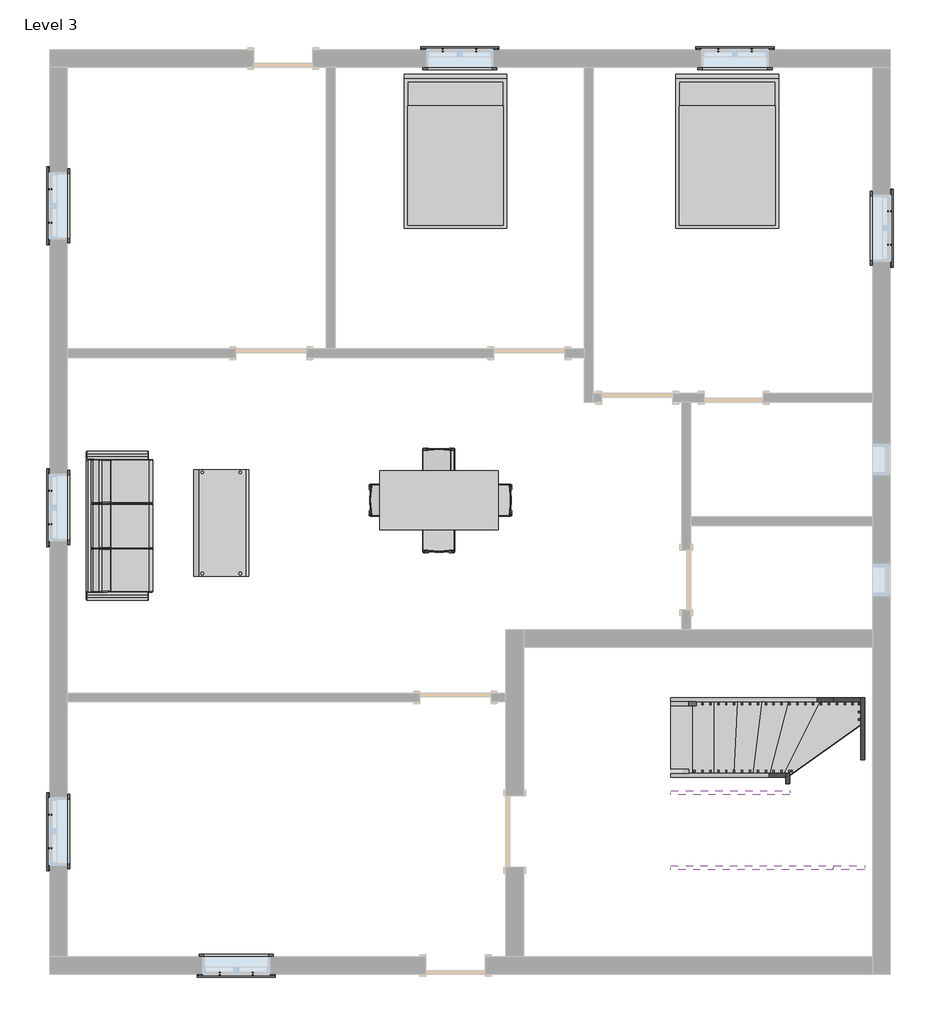
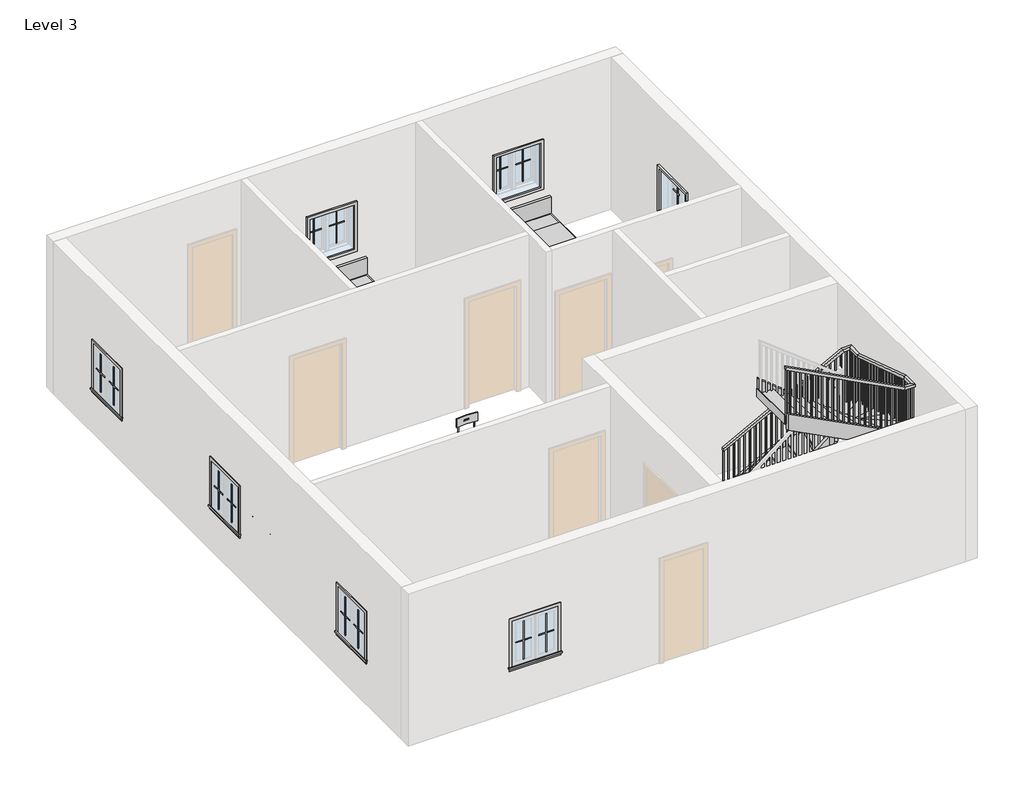
# One storey, part 2 of 2: 29 proxies, 8 members, 4 furniture elements, 1 railing, 1 stair flight.
"""IFC4 building model written with IfcOpenShell, lengths in millimetres."""

from ifc_helpers import new_model, si_unit, frame, origin, place, context, project, spatial, polyline, outline, extrude, faceted_brep, transform, mapped, element, save
from components import modern_coffee_table_17989_modern_coffee_table_17989_d3a860c8, muntin_pattern_2x2_muntin_pattern_2x2_b3fe6957, muntin_pattern_2x2_muntin_pattern_2x2_3e0ecaf2, trim_window_exterior_flat_with_sill_41619996, trim_window_interior_flat_picture_frame_51c85655, furniture_2fc85b74, furniture_29a9adb8, furniture_57072a26, bed_17739_bed_17739_15c61121, dining_table_w_chairs_11374_0cdfc61b, stair_flight_b9c50625

model = new_model("IFC4")

# Units and contexts
model_context = context("Model", 3, world=origin())
ifc_project = project(units=[si_unit("LENGTHUNIT", "METRE", prefix="MILLI")], contexts=[model_context])

# Site, building, storey
site = spatial("IfcSite", under=ifc_project)
building = spatial("IfcBuilding", under=site)
storey = spatial("IfcBuildingStorey", under=building, Name="Level 3", Elevation=3200.4)

# Proxies
placement = place(None, origin())
modern_coffee_table_17989_modern_coffee_table_17989_shape = modern_coffee_table_17989_modern_coffee_table_17989_d3a860c8(model_context)
element("IfcBuildingElementProxy", 1, Name="Modern_Coffee_Table_17989 : Modern_Coffee_Table_17989", ObjectType="Modern_Coffee_Table_17989 : Modern_Coffee_Table_17989", at=placement, inside=storey, context=model_context, shape_type="MappedRepresentation", body=[
    mapped(modern_coffee_table_17989_modern_coffee_table_17989_shape, transform((-4791.7841049, 1283.3840961, 3200.4), x_axis=(0.0, 1.0, 0.0), y_axis=(-1.0, 0.0, 0.0), z_axis=(0.0, 0.0, 1.0))),
])
muntin_pattern_2x2_muntin_pattern_2x2_shape = muntin_pattern_2x2_muntin_pattern_2x2_b3fe6957(model_context)
element("IfcBuildingElementProxy", 2, Name="Muntin Pattern_2x2 : Muntin Pattern_2x2", ObjectType="Muntin Pattern_2x2 : Muntin Pattern_2x2", at=placement, inside=storey, context=model_context, shape_type="MappedRepresentation", body=[
    mapped(muntin_pattern_2x2_muntin_pattern_2x2_shape, transform((-1586.7442864, 7129.6784997, 4184.65), x_axis=(1.0, 0.0, 0.0), y_axis=(0.0, 1.0, 0.0), z_axis=(0.0, 0.0, 1.0))),
])
element("IfcBuildingElementProxy", 3, Name="Muntin Pattern_2x2 : Muntin Pattern_2x2", ObjectType="Muntin Pattern_2x2 : Muntin Pattern_2x2", at=placement, inside=storey, context=model_context, shape_type="MappedRepresentation", body=[
    mapped(muntin_pattern_2x2_muntin_pattern_2x2_shape, transform((1952.1107136, 7129.6784997, 4184.65), x_axis=(1.0, 0.0, 0.0), y_axis=(0.0, 1.0, 0.0), z_axis=(0.0, 0.0, 1.0))),
])
element("IfcBuildingElementProxy", 4, Name="Muntin Pattern_2x2 : Muntin Pattern_2x2", ObjectType="Muntin Pattern_2x2 : Muntin Pattern_2x2", at=placement, inside=storey, context=model_context, shape_type="MappedRepresentation", body=[
    mapped(muntin_pattern_2x2_muntin_pattern_2x2_shape, transform((-6633.4067864, 4915.1159997, 4184.65), x_axis=(0.0, 1.0, 0.0), y_axis=(-1.0, 0.0, 0.0), z_axis=(0.0, 0.0, 1.0))),
])
element("IfcBuildingElementProxy", 5, Name="Muntin Pattern_2x2 : Muntin Pattern_2x2", ObjectType="Muntin Pattern_2x2 : Muntin Pattern_2x2", at=placement, inside=storey, context=model_context, shape_type="MappedRepresentation", body=[
    mapped(muntin_pattern_2x2_muntin_pattern_2x2_shape, transform((-6633.4067864, 1038.4409997, 4184.65), x_axis=(0.0, 1.0, 0.0), y_axis=(-1.0, 0.0, 0.0), z_axis=(0.0, 0.0, 1.0))),
])
element("IfcBuildingElementProxy", 6, Name="Muntin Pattern_2x2 : Muntin Pattern_2x2", ObjectType="Muntin Pattern_2x2 : Muntin Pattern_2x2", at=placement, inside=storey, context=model_context, shape_type="MappedRepresentation", body=[
    mapped(muntin_pattern_2x2_muntin_pattern_2x2_shape, transform((4152.7032136, 5057.9909997, 4184.65), x_axis=(0.0, -1.0, 0.0), y_axis=(1.0, 0.0, 0.0), z_axis=(0.0, 0.0, 1.0))),
])
element("IfcBuildingElementProxy", 7, Name="Muntin Pattern_2x2 : Muntin Pattern_2x2", ObjectType="Muntin Pattern_2x2 : Muntin Pattern_2x2", at=placement, inside=storey, context=model_context, shape_type="MappedRepresentation", body=[
    mapped(muntin_pattern_2x2_muntin_pattern_2x2_shape, transform((-6633.4067864, -3125.2540003, 4184.65), x_axis=(0.0, 1.0, 0.0), y_axis=(-1.0, 0.0, 0.0), z_axis=(0.0, 0.0, 1.0))),
])
element("IfcBuildingElementProxy", 8, Name="Muntin Pattern_2x2 : Muntin Pattern_2x2", ObjectType="Muntin Pattern_2x2 : Muntin Pattern_2x2", at=placement, inside=storey, context=model_context, shape_type="MappedRepresentation", body=[
    mapped(muntin_pattern_2x2_muntin_pattern_2x2_shape, transform((-4028.3192864, -4738.4715003, 4184.65), x_axis=(-1.0, 0.0, 0.0), y_axis=(0.0, -1.0, 0.0), z_axis=(0.0, 0.0, 1.0))),
])
muntin_pattern_2x2_muntin_pattern_2x2_2_shape = muntin_pattern_2x2_muntin_pattern_2x2_3e0ecaf2(model_context)
element("IfcBuildingElementProxy", 9, Name="Muntin Pattern_2x2 : Muntin Pattern_2x2", ObjectType="Muntin Pattern_2x2 : Muntin Pattern_2x2", at=placement, inside=storey, context=model_context, shape_type="MappedRepresentation", body=[
    mapped(muntin_pattern_2x2_muntin_pattern_2x2_2_shape, transform((-1158.1192864, 7129.6784997, 4184.65), x_axis=(-1.0, 0.0, 0.0), y_axis=(0.0, -1.0, 0.0), z_axis=(0.0, 0.0, 1.0))),
])
element("IfcBuildingElementProxy", 10, Name="Muntin Pattern_2x2 : Muntin Pattern_2x2", ObjectType="Muntin Pattern_2x2 : Muntin Pattern_2x2", at=placement, inside=storey, context=model_context, shape_type="MappedRepresentation", body=[
    mapped(muntin_pattern_2x2_muntin_pattern_2x2_2_shape, transform((2380.7357136, 7129.6784997, 4184.65), x_axis=(-1.0, 0.0, 0.0), y_axis=(0.0, -1.0, 0.0), z_axis=(0.0, 0.0, 1.0))),
])
element("IfcBuildingElementProxy", 11, Name="Muntin Pattern_2x2 : Muntin Pattern_2x2", ObjectType="Muntin Pattern_2x2 : Muntin Pattern_2x2", at=placement, inside=storey, context=model_context, shape_type="MappedRepresentation", body=[
    mapped(muntin_pattern_2x2_muntin_pattern_2x2_2_shape, transform((-6633.4067864, 5343.7409997, 4184.65), x_axis=(0.0, -1.0, 0.0), y_axis=(1.0, 0.0, 0.0), z_axis=(0.0, 0.0, 1.0))),
])
element("IfcBuildingElementProxy", 12, Name="Muntin Pattern_2x2 : Muntin Pattern_2x2", ObjectType="Muntin Pattern_2x2 : Muntin Pattern_2x2", at=placement, inside=storey, context=model_context, shape_type="MappedRepresentation", body=[
    mapped(muntin_pattern_2x2_muntin_pattern_2x2_2_shape, transform((-6633.4067864, 1467.0659997, 4184.65), x_axis=(0.0, -1.0, 0.0), y_axis=(1.0, 0.0, 0.0), z_axis=(0.0, 0.0, 1.0))),
])
element("IfcBuildingElementProxy", 13, Name="Muntin Pattern_2x2 : Muntin Pattern_2x2", ObjectType="Muntin Pattern_2x2 : Muntin Pattern_2x2", at=placement, inside=storey, context=model_context, shape_type="MappedRepresentation", body=[
    mapped(muntin_pattern_2x2_muntin_pattern_2x2_2_shape, transform((4152.7032136, 4629.3659997, 4184.65), x_axis=(0.0, 1.0, 0.0), y_axis=(-1.0, 0.0, 0.0), z_axis=(0.0, 0.0, 1.0))),
])
element("IfcBuildingElementProxy", 14, Name="Muntin Pattern_2x2 : Muntin Pattern_2x2", ObjectType="Muntin Pattern_2x2 : Muntin Pattern_2x2", at=placement, inside=storey, context=model_context, shape_type="MappedRepresentation", body=[
    mapped(muntin_pattern_2x2_muntin_pattern_2x2_2_shape, transform((-6633.4067864, -2696.6290003, 4184.65), x_axis=(0.0, -1.0, 0.0), y_axis=(1.0, 0.0, 0.0), z_axis=(0.0, 0.0, 1.0))),
])
element("IfcBuildingElementProxy", 15, Name="Muntin Pattern_2x2 : Muntin Pattern_2x2", ObjectType="Muntin Pattern_2x2 : Muntin Pattern_2x2", at=placement, inside=storey, context=model_context, shape_type="MappedRepresentation", body=[
    mapped(muntin_pattern_2x2_muntin_pattern_2x2_2_shape, transform((-4456.9442864, -4738.4715003, 4184.65), x_axis=(1.0, 0.0, 0.0), y_axis=(0.0, 1.0, 0.0), z_axis=(0.0, 0.0, 1.0))),
])
trim_window_exterior_flat_with_sill_shape = trim_window_exterior_flat_with_sill_41619996(model_context)
element("IfcBuildingElementProxy", 16, Name="Trim-Window-Exterior-Flat : with Sill", ObjectType="Trim-Window-Exterior-Flat : with Sill", at=placement, inside=storey, context=model_context, shape_type="MappedRepresentation", body=[
    mapped(trim_window_exterior_flat_with_sill_shape, transform((-1372.4317864, 7139.2034997, 5029.2), x_axis=(-1.0, 0.0, 0.0), y_axis=(0.0, 0.0, 1.0), z_axis=(0.0, 1.0, 0.0))),
])
element("IfcBuildingElementProxy", 17, Name="Trim-Window-Exterior-Flat : with Sill", ObjectType="Trim-Window-Exterior-Flat : with Sill", at=placement, inside=storey, context=model_context, shape_type="MappedRepresentation", body=[
    mapped(trim_window_exterior_flat_with_sill_shape, transform((2166.4232136, 7139.2034997, 5029.2), x_axis=(-1.0, 0.0, 0.0), y_axis=(0.0, 0.0, 1.0), z_axis=(0.0, 1.0, 0.0))),
])
element("IfcBuildingElementProxy", 18, Name="Trim-Window-Exterior-Flat : with Sill", ObjectType="Trim-Window-Exterior-Flat : with Sill", at=placement, inside=storey, context=model_context, shape_type="MappedRepresentation", body=[
    mapped(trim_window_exterior_flat_with_sill_shape, transform((-6642.9317864, 5129.4284997, 5029.2), x_axis=(0.0, -1.0, 0.0), y_axis=(0.0, 0.0, 1.0), z_axis=(-1.0, 0.0, 0.0))),
])
element("IfcBuildingElementProxy", 19, Name="Trim-Window-Exterior-Flat : with Sill", ObjectType="Trim-Window-Exterior-Flat : with Sill", at=placement, inside=storey, context=model_context, shape_type="MappedRepresentation", body=[
    mapped(trim_window_exterior_flat_with_sill_shape, transform((-6642.9317864, 1252.7534997, 5029.2), x_axis=(0.0, -1.0, 0.0), y_axis=(0.0, 0.0, 1.0), z_axis=(-1.0, 0.0, 0.0))),
])
element("IfcBuildingElementProxy", 20, Name="Trim-Window-Exterior-Flat : with Sill", ObjectType="Trim-Window-Exterior-Flat : with Sill", at=placement, inside=storey, context=model_context, shape_type="MappedRepresentation", body=[
    mapped(trim_window_exterior_flat_with_sill_shape, transform((4162.2282136, 4843.6784997, 5029.2), x_axis=(0.0, 1.0, 0.0), y_axis=(0.0, 0.0, 1.0), z_axis=(1.0, 0.0, 0.0))),
])
element("IfcBuildingElementProxy", 21, Name="Trim-Window-Exterior-Flat : with Sill", ObjectType="Trim-Window-Exterior-Flat : with Sill", at=placement, inside=storey, context=model_context, shape_type="MappedRepresentation", body=[
    mapped(trim_window_exterior_flat_with_sill_shape, transform((-6642.9317864, -2910.9415003, 5029.2), x_axis=(0.0, -1.0, 0.0), y_axis=(0.0, 0.0, 1.0), z_axis=(-1.0, 0.0, 0.0))),
])
element("IfcBuildingElementProxy", 22, Name="Trim-Window-Exterior-Flat : with Sill", ObjectType="Trim-Window-Exterior-Flat : with Sill", at=placement, inside=storey, context=model_context, shape_type="MappedRepresentation", body=[
    mapped(trim_window_exterior_flat_with_sill_shape, transform((-4242.6317864, -4747.9965003, 5029.2), x_axis=(1.0, 0.0, 0.0), y_axis=(0.0, 0.0, 1.0), z_axis=(0.0, -1.0, 0.0))),
])
trim_window_interior_flat_picture_frame_shape = trim_window_interior_flat_picture_frame_51c85655(model_context)
element("IfcBuildingElementProxy", 23, Name="Trim-Window-Interior-Flat : Picture Frame", ObjectType="Trim-Window-Interior-Flat : Picture Frame", at=placement, inside=storey, context=model_context, shape_type="MappedRepresentation", body=[
    mapped(trim_window_interior_flat_picture_frame_shape, transform((-1372.4317864, 6910.6034997, 5029.2), x_axis=(1.0, 0.0, 0.0), y_axis=(0.0, 0.0, 1.0), z_axis=(0.0, -1.0, 0.0))),
])
element("IfcBuildingElementProxy", 24, Name="Trim-Window-Interior-Flat : Picture Frame", ObjectType="Trim-Window-Interior-Flat : Picture Frame", at=placement, inside=storey, context=model_context, shape_type="MappedRepresentation", body=[
    mapped(trim_window_interior_flat_picture_frame_shape, transform((2166.4232136, 6910.6034997, 5029.2), x_axis=(1.0, 0.0, 0.0), y_axis=(0.0, 0.0, 1.0), z_axis=(0.0, -1.0, 0.0))),
])
element("IfcBuildingElementProxy", 25, Name="Trim-Window-Interior-Flat : Picture Frame", ObjectType="Trim-Window-Interior-Flat : Picture Frame", at=placement, inside=storey, context=model_context, shape_type="MappedRepresentation", body=[
    mapped(trim_window_interior_flat_picture_frame_shape, transform((-6414.3317864, 5129.4284997, 5029.2), x_axis=(0.0, 1.0, 0.0), y_axis=(0.0, 0.0, 1.0), z_axis=(1.0, 0.0, 0.0))),
])
element("IfcBuildingElementProxy", 26, Name="Trim-Window-Interior-Flat : Picture Frame", ObjectType="Trim-Window-Interior-Flat : Picture Frame", at=placement, inside=storey, context=model_context, shape_type="MappedRepresentation", body=[
    mapped(trim_window_interior_flat_picture_frame_shape, transform((-6414.3317864, 1252.7534997, 5029.2), x_axis=(0.0, 1.0, 0.0), y_axis=(0.0, 0.0, 1.0), z_axis=(1.0, 0.0, 0.0))),
])
element("IfcBuildingElementProxy", 27, Name="Trim-Window-Interior-Flat : Picture Frame", ObjectType="Trim-Window-Interior-Flat : Picture Frame", at=placement, inside=storey, context=model_context, shape_type="MappedRepresentation", body=[
    mapped(trim_window_interior_flat_picture_frame_shape, transform((3933.6282136, 4843.6784997, 5029.2), x_axis=(0.0, -1.0, 0.0), y_axis=(0.0, 0.0, 1.0), z_axis=(-1.0, 0.0, 0.0))),
])
element("IfcBuildingElementProxy", 28, Name="Trim-Window-Interior-Flat : Picture Frame", ObjectType="Trim-Window-Interior-Flat : Picture Frame", at=placement, inside=storey, context=model_context, shape_type="MappedRepresentation", body=[
    mapped(trim_window_interior_flat_picture_frame_shape, transform((-6414.3317864, -2910.9415003, 5029.2), x_axis=(0.0, 1.0, 0.0), y_axis=(0.0, 0.0, 1.0), z_axis=(1.0, 0.0, 0.0))),
])
element("IfcBuildingElementProxy", 29, Name="Trim-Window-Interior-Flat : Picture Frame", ObjectType="Trim-Window-Interior-Flat : Picture Frame", at=placement, inside=storey, context=model_context, shape_type="MappedRepresentation", body=[
    mapped(trim_window_interior_flat_picture_frame_shape, transform((-4242.6317864, -4519.3965003, 5029.2), x_axis=(-1.0, 0.0, 0.0), y_axis=(0.0, 0.0, 1.0), z_axis=(0.0, 1.0, 0.0))),
])

# Furniture
furniture_shape = furniture_2fc85b74(model_context)
furniture_2_shape = furniture_29a9adb8(model_context)
furniture_3_shape = furniture_57072a26(model_context)
element("IfcFurniture", 30, at=placement, inside=storey, context=model_context, shape_type="MappedRepresentation", body=[
    mapped(furniture_shape, transform((-5371.0104604, 1017.8034997, 3200.4), x_axis=(0.0, 1.0, 0.0), y_axis=(-1.0, 0.0, 0.0), z_axis=(0.0, 0.0, 1.0))),
    mapped(furniture_2_shape, transform((-5371.0104604, 1017.8034997, 3200.4), x_axis=(0.0, 1.0, 0.0), y_axis=(-1.0, 0.0, 0.0), z_axis=(0.0, 0.0, 1.0))),
    mapped(furniture_3_shape, transform((-5371.0104604, 1017.8034997, 3200.4), x_axis=(0.0, 1.0, 0.0), y_axis=(-1.0, 0.0, 0.0), z_axis=(0.0, 0.0, 1.0))),
])
bed_17739_bed_17739_shape = bed_17739_bed_17739_15c61121(model_context)
element("IfcFurniture", 31, ObjectType="Bed_17739 : Bed_17739", at=placement, inside=storey, context=model_context, shape_type="MappedRepresentation", body=[
    mapped(bed_17739_bed_17739_shape, transform((-1425.7717864, 5805.7034997, 3200.4), x_axis=(1.0, 0.0, 0.0), y_axis=(0.0, 1.0, 0.0), z_axis=(0.0, 0.0, 1.0))),
])
element("IfcFurniture", 32, ObjectType="Bed_17739 : Bed_17739", at=placement, inside=storey, context=model_context, shape_type="MappedRepresentation", body=[
    mapped(bed_17739_bed_17739_shape, transform((2066.7282136, 5805.7034997, 3200.4), x_axis=(1.0, 0.0, 0.0), y_axis=(0.0, 1.0, 0.0), z_axis=(0.0, 0.0, 1.0))),
])
dining_table_w_chairs_11374_shape = dining_table_w_chairs_11374_0cdfc61b(model_context)
element("IfcFurniture", 33, ObjectType="Dining_Table_w_Chairs_11374", at=placement, inside=storey, context=model_context, shape_type="MappedRepresentation", body=[
    mapped(dining_table_w_chairs_11374_shape, transform((-1657.0397106, 1252.0888157, 3200.4), x_axis=(1.0, 0.0, 0.0), y_axis=(0.0, 1.0, 0.0), z_axis=(0.0, 0.0, 1.0))),
])

# Members
element("IfcMember", 34, ObjectType="Stringer - 2\" Width", at=placement, inside=storey, context=model_context, shape_type="SweptSolid", body=[
    extrude(outline(polyline([(3430.039954, 1342.8282136), (3200.4, 1342.8282136), (3200.4, 1562.5905312), (4162.900629, 3430.2454053), (4505.7956453, 3430.2454053), (3430.039954, 1342.8282136)])), frame((0.0, -1245.3365003, 0.0), z_axis=(0.0, 1.0, 0.0), x_axis=(0.0, 0.0, 1.0)), (0.0, 0.0, 1.0), 50.8),
])
element("IfcMember", 35, ObjectType="Stringer - 2\" Width", at=placement, inside=storey, context=model_context, shape_type="SweptSolid", body=[
    extrude(outline(polyline([(3430.2454053, -1245.3365003), (3430.2454053, -1194.5365003), (3784.9599055, -1194.5365003), (3784.9599055, -1245.3365003), (3430.2454053, -1245.3365003)])), frame((0.0, 0.0, 4162.900629), z_axis=(0.0, 0.0, 1.0), x_axis=(1.0, 0.0, 0.0)), (0.0, 0.0, 1.0), 342.8950162),
])
element("IfcMember", 36, ObjectType="Stringer - 2\" Width", at=placement, inside=storey, context=model_context, shape_type="SweptSolid", body=[
    extrude(outline(polyline([(-1194.5365003, 4489.4952212), (-1194.5365003, 4200.9956453), (-1364.0589833, 4200.9956453), (-3353.5365003, 4839.3682298), (-3353.5365003, 5170.3972697), (-3316.5563831, 5170.3972697), (-1194.5365003, 4489.4952212)])), frame((3784.9599055, 0.0, 0.0), z_axis=(1.0, 0.0, 0.0), x_axis=(0.0, 1.0, 0.0)), (0.0, 0.0, 1.0), 50.8),
])
element("IfcMember", 37, ObjectType="Stringer - 2\" Width", at=placement, inside=storey, context=model_context, shape_type="SweptSolid", body=[
    extrude(outline(polyline([(3835.7599055, -3353.5365003), (3835.7599055, -3404.3365003), (3430.2454053, -3404.3365003), (3430.2454053, -3353.5365003), (3835.7599055, -3353.5365003)])), frame((0.0, 0.0, 4850.2904473), z_axis=(0.0, 0.0, 1.0), x_axis=(1.0, 0.0, 0.0)), (0.0, 0.0, 1.0), 320.1068224),
])
element("IfcMember", 38, ObjectType="Stringer - 2\" Width", at=placement, inside=storey, context=model_context, shape_type="SweptSolid", body=[
    extrude(outline(polyline([(4850.2904473, 3430.2454053), (5170.3972697, 3430.2454053), (6246.1529609, 1342.8282136), (5926.0461385, 1342.8282136), (4850.2904473, 3430.2454053)])), frame((0.0, -3404.3365003, 0.0), z_axis=(0.0, 1.0, 0.0), x_axis=(0.0, 0.0, 1.0)), (0.0, 0.0, 1.0), 50.8),
])
element("IfcMember", 39, ObjectType="Stringer - 2\" Width", at=placement, inside=storey, context=model_context, shape_type="SweptSolid", body=[
    extrude(outline(polyline([(3376.5764461, 1342.8282136), (3200.4, 1342.8282136), (3200.4, 1609.0898582), (4187.5410923, 2819.7599055), (4580.818648, 2819.7599055), (3376.5764461, 1342.8282136)])), frame((0.0, -2210.5365003, 0.0), z_axis=(0.0, 1.0, 0.0), x_axis=(0.0, 0.0, 1.0)), (0.0, 0.0, 1.0), 50.8),
])
element("IfcMember", 40, ObjectType="Stringer - 2\" Width", at=placement, inside=storey, context=model_context, shape_type="SweptSolid", body=[
    extrude(outline(polyline([(-2159.7365003, 4773.6682978), (-2159.7365003, 4228.9617647), (-2193.9787177, 4228.9617647), (-2388.3365003, 4560.865107), (-2388.3365003, 5126.5409689), (-2366.3736178, 5126.5409689), (-2159.7365003, 4773.6682978)])), frame((2819.7599055, 0.0, 0.0), z_axis=(1.0, 0.0, 0.0), x_axis=(0.0, 1.0, 0.0)), (0.0, 0.0, 1.0), 50.8),
])
element("IfcMember", 41, ObjectType="Stringer - 2\" Width", at=placement, inside=storey, context=model_context, shape_type="SweptSolid", body=[
    extrude(outline(polyline([(4733.2634131, 2870.5599055), (5126.5409689, 2870.5599055), (6372.2038432, 1342.8282136), (5978.9262875, 1342.8282136), (4733.2634131, 2870.5599055)])), frame((0.0, -2439.1365003, 0.0), z_axis=(0.0, 1.0, 0.0), x_axis=(0.0, 0.0, 1.0)), (0.0, 0.0, 1.0), 50.8),
])

# Railing
element("IfcRailing", 42, ObjectType="Handrail - Rectangular", at=placement, inside=storey, context=model_context, shape_type="SolidModel", body=[
    faceted_brep([(1342.8282136, -1245.3365003, 4284.1333333), (1342.8282136, -1245.3365003, 4226.6742652), (1342.8282136, -1296.1365003, 4226.6742652), (1342.8282136, -1296.1365003, 4284.1333333), (3600.5532757, -1245.3365003, 5477.4239201), (3613.1523402, -1245.3365003, 5426.6239201), (3613.1523402, -1296.1365003, 5426.6239201), (3600.5532757, -1296.1365003, 5477.4239201), (3784.9599055, -1245.3365003, 5477.4239201), (3784.9599055, -1245.3365003, 5426.6239201), (3734.1599055, -1296.1365003, 5426.6239201), (3734.1599055, -1296.1365003, 5477.4239201), (3784.9599055, -1532.6483825, 5477.4239201), (3784.9599055, -1540.5989586, 5426.6239201), (3734.1599055, -1540.5989586, 5426.6239201), (3734.1599055, -1532.6483825, 5477.4239201), (3784.9599055, -3066.2246182, 5969.5094132), (3784.9599055, -3074.1751943, 5918.7094132), (3734.1599055, -3074.1751943, 5918.7094132), (3734.1599055, -3066.2246182, 5969.5094132), (3784.9599055, -3353.5365003, 5969.5094132), (3784.9599055, -3353.5365003, 5918.7094132), (3734.1599055, -3302.7365003, 5918.7094132), (3734.1599055, -3302.7365003, 5969.5094132), (3600.5532757, -3353.5365003, 5969.5094132), (3587.9542112, -3353.5365003, 5918.7094132), (3587.9542112, -3302.7365003, 5918.7094132), (3600.5532757, -3302.7365003, 5969.5094132), (1342.8282136, -3353.5365003, 7162.8), (1342.8282136, -3302.7365003, 7162.8), (1342.8282136, -3302.7365003, 7105.3409318), (1342.8282136, -3353.5365003, 7105.3409318)], [[[0, 1, 2, 3]], [[1, 0, 4, 5]], [[2, 1, 5, 6]], [[3, 2, 6, 7]], [[0, 3, 7, 4]], [[5, 4, 8, 9]], [[6, 5, 9, 10]], [[7, 6, 10, 11]], [[4, 7, 11, 8]], [[9, 8, 12, 13]], [[10, 9, 13, 14]], [[11, 10, 14, 15]], [[8, 11, 15, 12]], [[13, 12, 16, 17]], [[14, 13, 17, 18]], [[15, 14, 18, 19]], [[12, 15, 19, 16]], [[17, 16, 20, 21]], [[18, 17, 21, 22]], [[19, 18, 22, 23]], [[16, 19, 23, 20]], [[21, 20, 24, 25]], [[22, 21, 25, 26]], [[23, 22, 26, 27]], [[20, 23, 27, 24]], [[28, 29, 30, 31]], [[25, 24, 28, 31]], [[26, 25, 31, 30]], [[27, 26, 30, 29]], [[24, 27, 29, 28]]]),
    extrude(outline(polyline([(7068.1284102, 1413.2349055), (6079.0666667, 1413.2349055), (6079.0666667, 1432.2849055), (7058.0597858, 1432.2849055), (7068.1284102, 1413.2349055)])), frame((0.0, -3337.6615003, 0.0), z_axis=(0.0, 1.0, 0.0), x_axis=(0.0, 0.0, 1.0)), (0.0, 0.0, 1.0), 19.05),
    extrude(outline(polyline([(7014.42908, 1514.8349055), (6079.0666667, 1514.8349055), (6079.0666667, 1533.8849055), (7004.3604556, 1533.8849055), (7014.42908, 1514.8349055)])), frame((0.0, -3337.6615003, 0.0), z_axis=(0.0, 1.0, 0.0), x_axis=(0.0, 0.0, 1.0)), (0.0, 0.0, 1.0), 19.05),
    extrude(outline(polyline([(6960.7297498, 1616.4349055), (5909.7333333, 1616.4349055), (5909.7333333, 1635.4849055), (6950.6611254, 1635.4849055), (6960.7297498, 1616.4349055)])), frame((0.0, -3337.6615003, 0.0), z_axis=(0.0, 1.0, 0.0), x_axis=(0.0, 0.0, 1.0)), (0.0, 0.0, 1.0), 19.05),
    extrude(outline(polyline([(6907.0304196, 1718.0349055), (5909.7333333, 1718.0349055), (5909.7333333, 1737.0849055), (6896.9617952, 1737.0849055), (6907.0304196, 1718.0349055)])), frame((0.0, -3337.6615003, 0.0), z_axis=(0.0, 1.0, 0.0), x_axis=(0.0, 0.0, 1.0)), (0.0, 0.0, 1.0), 19.05),
    extrude(outline(polyline([(6853.3310894, 1819.6349055), (5909.7333333, 1819.6349055), (5909.7333333, 1838.6849055), (6843.262465, 1838.6849055), (6853.3310894, 1819.6349055)])), frame((0.0, -3337.6615003, 0.0), z_axis=(0.0, 1.0, 0.0), x_axis=(0.0, 0.0, 1.0)), (0.0, 0.0, 1.0), 19.05),
    extrude(outline(polyline([(6799.6317592, 1921.2349055), (5740.4, 1921.2349055), (5740.4, 1940.2849055), (6789.5631348, 1940.2849055), (6799.6317592, 1921.2349055)])), frame((0.0, -3337.6615003, 0.0), z_axis=(0.0, 1.0, 0.0), x_axis=(0.0, 0.0, 1.0)), (0.0, 0.0, 1.0), 19.05),
    extrude(outline(polyline([(6745.932429, 2022.8349055), (5740.4, 2022.8349055), (5740.4, 2041.8849055), (6735.8638046, 2041.8849055), (6745.932429, 2022.8349055)])), frame((0.0, -3337.6615003, 0.0), z_axis=(0.0, 1.0, 0.0), x_axis=(0.0, 0.0, 1.0)), (0.0, 0.0, 1.0), 19.05),
    extrude(outline(polyline([(6692.2330988, 2124.4349055), (5740.4, 2124.4349055), (5740.4, 2143.4849055), (6682.1644744, 2143.4849055), (6692.2330988, 2124.4349055)])), frame((0.0, -3337.6615003, 0.0), z_axis=(0.0, 1.0, 0.0), x_axis=(0.0, 0.0, 1.0)), (0.0, 0.0, 1.0), 19.05),
    extrude(outline(polyline([(6638.5337686, 2226.0349055), (5571.0666667, 2226.0349055), (5571.0666667, 2245.0849055), (6628.4651442, 2245.0849055), (6638.5337686, 2226.0349055)])), frame((0.0, -3337.6615003, 0.0), z_axis=(0.0, 1.0, 0.0), x_axis=(0.0, 0.0, 1.0)), (0.0, 0.0, 1.0), 19.05),
    extrude(outline(polyline([(6584.8344384, 2327.6349055), (5571.0666667, 2327.6349055), (5571.0666667, 2346.6849055), (6574.765814, 2346.6849055), (6584.8344384, 2327.6349055)])), frame((0.0, -3337.6615003, 0.0), z_axis=(0.0, 1.0, 0.0), x_axis=(0.0, 0.0, 1.0)), (0.0, 0.0, 1.0), 19.05),
    extrude(outline(polyline([(6531.1351082, 2429.2349055), (5571.0666667, 2429.2349055), (5571.0666667, 2448.2849055), (6521.0664838, 2448.2849055), (6531.1351082, 2429.2349055)])), frame((0.0, -3337.6615003, 0.0), z_axis=(0.0, 1.0, 0.0), x_axis=(0.0, 0.0, 1.0)), (0.0, 0.0, 1.0), 19.05),
    extrude(outline(polyline([(6477.435778, 2530.8349055), (5401.7333333, 2530.8349055), (5401.7333333, 2549.8849055), (6467.3671536, 2549.8849055), (6477.435778, 2530.8349055)])), frame((0.0, -3337.6615003, 0.0), z_axis=(0.0, 1.0, 0.0), x_axis=(0.0, 0.0, 1.0)), (0.0, 0.0, 1.0), 19.05),
    extrude(outline(polyline([(6423.7364478, 2632.4349055), (5401.7333333, 2632.4349055), (5401.7333333, 2651.4849055), (6413.6678234, 2651.4849055), (6423.7364478, 2632.4349055)])), frame((0.0, -3337.6615003, 0.0), z_axis=(0.0, 1.0, 0.0), x_axis=(0.0, 0.0, 1.0)), (0.0, 0.0, 1.0), 19.05),
    extrude(outline(polyline([(6370.0371176, 2734.0349055), (5401.7333333, 2734.0349055), (5401.7333333, 2753.0849055), (6359.9684932, 2753.0849055), (6370.0371176, 2734.0349055)])), frame((0.0, -3337.6615003, 0.0), z_axis=(0.0, 1.0, 0.0), x_axis=(0.0, 0.0, 1.0)), (0.0, 0.0, 1.0), 19.05),
    extrude(outline(polyline([(6316.3377874, 2835.6349055), (5401.7333333, 2835.6349055), (5401.7333333, 2854.6849055), (6306.269163, 2854.6849055), (6316.3377874, 2835.6349055)])), frame((0.0, -3337.6615003, 0.0), z_axis=(0.0, 1.0, 0.0), x_axis=(0.0, 0.0, 1.0)), (0.0, 0.0, 1.0), 19.05),
    extrude(outline(polyline([(6262.6384572, 2937.2349055), (5232.4, 2937.2349055), (5232.4, 2956.2849055), (6252.5698328, 2956.2849055), (6262.6384572, 2937.2349055)])), frame((0.0, -3337.6615003, 0.0), z_axis=(0.0, 1.0, 0.0), x_axis=(0.0, 0.0, 1.0)), (0.0, 0.0, 1.0), 19.05),
    extrude(outline(polyline([(6208.939127, 3038.8349055), (5232.4, 3038.8349055), (5232.4, 3057.8849055), (6198.8705026, 3057.8849055), (6208.939127, 3038.8349055)])), frame((0.0, -3337.6615003, 0.0), z_axis=(0.0, 1.0, 0.0), x_axis=(0.0, 0.0, 1.0)), (0.0, 0.0, 1.0), 19.05),
    extrude(outline(polyline([(6155.2397968, 3140.4349055), (5232.4, 3140.4349055), (5232.4, 3159.4849055), (6145.1711724, 3159.4849055), (6155.2397968, 3140.4349055)])), frame((0.0, -3337.6615003, 0.0), z_axis=(0.0, 1.0, 0.0), x_axis=(0.0, 0.0, 1.0)), (0.0, 0.0, 1.0), 19.05),
    extrude(outline(polyline([(6101.5404666, 3242.0349055), (5232.4, 3242.0349055), (5232.4, 3261.0849055), (6091.4718422, 3261.0849055), (6101.5404666, 3242.0349055)])), frame((0.0, -3337.6615003, 0.0), z_axis=(0.0, 1.0, 0.0), x_axis=(0.0, 0.0, 1.0)), (0.0, 0.0, 1.0), 19.05),
    extrude(outline(polyline([(6047.8411364, 3343.6349055), (5063.0666667, 3343.6349055), (5063.0666667, 3362.6849055), (6037.772512, 3362.6849055), (6047.8411364, 3343.6349055)])), frame((0.0, -3337.6615003, 0.0), z_axis=(0.0, 1.0, 0.0), x_axis=(0.0, 0.0, 1.0)), (0.0, 0.0, 1.0), 19.05),
    extrude(outline(polyline([(5994.1418062, 3445.2349055), (5063.0666667, 3445.2349055), (5063.0666667, 3464.2849055), (5984.0731818, 3464.2849055), (5994.1418062, 3445.2349055)])), frame((0.0, -3337.6615003, 0.0), z_axis=(0.0, 1.0, 0.0), x_axis=(0.0, 0.0, 1.0)), (0.0, 0.0, 1.0), 19.05),
    extrude(outline(polyline([(5940.442476, 3546.8349055), (5063.0666667, 3546.8349055), (5063.0666667, 3565.8849055), (5930.3738516, 3565.8849055), (5940.442476, 3546.8349055)])), frame((0.0, -3337.6615003, 0.0), z_axis=(0.0, 1.0, 0.0), x_axis=(0.0, 0.0, 1.0)), (0.0, 0.0, 1.0), 19.05),
    extrude(outline(polyline([(3667.4849055, -3337.6615003), (3648.4349055, -3337.6615003), (3648.4349055, -3318.6115003), (3667.4849055, -3318.6115003), (3667.4849055, -3337.6615003)])), frame((0.0, 0.0, 5063.0666667), z_axis=(0.0, 0.0, 1.0), x_axis=(1.0, 0.0, 0.0)), (0.0, 0.0, 1.0), 855.6427466),
    extrude(outline(polyline([(3769.0849055, -3293.2115003), (3769.0849055, -3312.2615003), (3750.0349055, -3312.2615003), (3750.0349055, -3293.2115003), (3769.0849055, -3293.2115003)])), frame((0.0, 0.0, 5063.0666667), z_axis=(0.0, 0.0, 1.0), x_axis=(1.0, 0.0, 0.0)), (0.0, 0.0, 1.0), 855.6427466),
    extrude(outline(polyline([(3769.0849055, -3191.6115003), (3769.0849055, -3210.6615003), (3750.0349055, -3210.6615003), (3750.0349055, -3191.6115003), (3769.0849055, -3191.6115003)])), frame((0.0, 0.0, 5063.0666667), z_axis=(0.0, 0.0, 1.0), x_axis=(1.0, 0.0, 0.0)), (0.0, 0.0, 1.0), 855.6427466),
    extrude(outline(polyline([(3769.0849055, -3090.0115003), (3769.0849055, -3109.0615003), (3750.0349055, -3109.0615003), (3750.0349055, -3090.0115003), (3769.0849055, -3090.0115003)])), frame((0.0, 0.0, 5063.0666667), z_axis=(0.0, 0.0, 1.0), x_axis=(1.0, 0.0, 0.0)), (0.0, 0.0, 1.0), 855.6427466),
    extrude(outline(polyline([(-2988.4115003, 5891.1900316), (-2988.4115003, 4893.7333333), (-3007.4615003, 4893.7333333), (-3007.4615003, 5897.3026907), (-2988.4115003, 5891.1900316)])), frame((3750.0349055, 0.0, 0.0), z_axis=(1.0, 0.0, 0.0), x_axis=(0.0, 1.0, 0.0)), (0.0, 0.0, 1.0), 19.05),
    extrude(outline(polyline([(-2886.8115003, 5858.5891834), (-2886.8115003, 4893.7333333), (-2905.8615003, 4893.7333333), (-2905.8615003, 5864.7018425), (-2886.8115003, 5858.5891834)])), frame((3750.0349055, 0.0, 0.0), z_axis=(1.0, 0.0, 0.0), x_axis=(0.0, 1.0, 0.0)), (0.0, 0.0, 1.0), 19.05),
    extrude(outline(polyline([(-2785.2115003, 5825.9883352), (-2785.2115003, 4893.7333333), (-2804.2615003, 4893.7333333), (-2804.2615003, 5832.1009942), (-2785.2115003, 5825.9883352)])), frame((3750.0349055, 0.0, 0.0), z_axis=(1.0, 0.0, 0.0), x_axis=(0.0, 1.0, 0.0)), (0.0, 0.0, 1.0), 19.05),
    extrude(outline(polyline([(-2683.6115003, 5793.387487), (-2683.6115003, 4893.7333333), (-2702.6615003, 4893.7333333), (-2702.6615003, 5799.500146), (-2683.6115003, 5793.387487)])), frame((3750.0349055, 0.0, 0.0), z_axis=(1.0, 0.0, 0.0), x_axis=(0.0, 1.0, 0.0)), (0.0, 0.0, 1.0), 19.05),
    extrude(outline(polyline([(-2582.0115003, 5760.7866387), (-2582.0115003, 4893.7333333), (-2601.0615003, 4893.7333333), (-2601.0615003, 5766.8992978), (-2582.0115003, 5760.7866387)])), frame((3750.0349055, 0.0, 0.0), z_axis=(1.0, 0.0, 0.0), x_axis=(0.0, 1.0, 0.0)), (0.0, 0.0, 1.0), 19.05),
    extrude(outline(polyline([(-2480.4115003, 5728.1857905), (-2480.4115003, 4724.4), (-2499.4615003, 4724.4), (-2499.4615003, 5734.2984495), (-2480.4115003, 5728.1857905)])), frame((3750.0349055, 0.0, 0.0), z_axis=(1.0, 0.0, 0.0), x_axis=(0.0, 1.0, 0.0)), (0.0, 0.0, 1.0), 19.05),
    extrude(outline(polyline([(-2378.8115003, 5695.5849423), (-2378.8115003, 4724.4), (-2397.8615003, 4724.4), (-2397.8615003, 5701.6976013), (-2378.8115003, 5695.5849423)])), frame((3750.0349055, 0.0, 0.0), z_axis=(1.0, 0.0, 0.0), x_axis=(0.0, 1.0, 0.0)), (0.0, 0.0, 1.0), 19.05),
    extrude(outline(polyline([(-2277.2115003, 5662.984094), (-2277.2115003, 4724.4), (-2296.2615003, 4724.4), (-2296.2615003, 5669.0967531), (-2277.2115003, 5662.984094)])), frame((3750.0349055, 0.0, 0.0), z_axis=(1.0, 0.0, 0.0), x_axis=(0.0, 1.0, 0.0)), (0.0, 0.0, 1.0), 19.05),
    extrude(outline(polyline([(-2175.6115003, 5630.3832458), (-2175.6115003, 4724.4), (-2194.6615003, 4724.4), (-2194.6615003, 5636.4959049), (-2175.6115003, 5630.3832458)])), frame((3750.0349055, 0.0, 0.0), z_axis=(1.0, 0.0, 0.0), x_axis=(0.0, 1.0, 0.0)), (0.0, 0.0, 1.0), 19.05),
    extrude(outline(polyline([(-2074.0115003, 5597.7823976), (-2074.0115003, 4724.4), (-2093.0615003, 4724.4), (-2093.0615003, 5603.8950566), (-2074.0115003, 5597.7823976)])), frame((3750.0349055, 0.0, 0.0), z_axis=(1.0, 0.0, 0.0), x_axis=(0.0, 1.0, 0.0)), (0.0, 0.0, 1.0), 19.05),
    extrude(outline(polyline([(-1972.4115003, 5565.1815494), (-1972.4115003, 4555.0666667), (-1991.4615003, 4555.0666667), (-1991.4615003, 5571.2942084), (-1972.4115003, 5565.1815494)])), frame((3750.0349055, 0.0, 0.0), z_axis=(1.0, 0.0, 0.0), x_axis=(0.0, 1.0, 0.0)), (0.0, 0.0, 1.0), 19.05),
    extrude(outline(polyline([(-1870.8115003, 5532.5807011), (-1870.8115003, 4555.0666667), (-1889.8615003, 4555.0666667), (-1889.8615003, 5538.6933602), (-1870.8115003, 5532.5807011)])), frame((3750.0349055, 0.0, 0.0), z_axis=(1.0, 0.0, 0.0), x_axis=(0.0, 1.0, 0.0)), (0.0, 0.0, 1.0), 19.05),
    extrude(outline(polyline([(-1769.2115003, 5499.9798529), (-1769.2115003, 4555.0666667), (-1788.2615003, 4555.0666667), (-1788.2615003, 5506.092512), (-1769.2115003, 5499.9798529)])), frame((3750.0349055, 0.0, 0.0), z_axis=(1.0, 0.0, 0.0), x_axis=(0.0, 1.0, 0.0)), (0.0, 0.0, 1.0), 19.05),
    extrude(outline(polyline([(-1667.6115003, 5467.3790047), (-1667.6115003, 4555.0666667), (-1686.6615003, 4555.0666667), (-1686.6615003, 5473.4916637), (-1667.6115003, 5467.3790047)])), frame((3750.0349055, 0.0, 0.0), z_axis=(1.0, 0.0, 0.0), x_axis=(0.0, 1.0, 0.0)), (0.0, 0.0, 1.0), 19.05),
    extrude(outline(polyline([(-1566.0115003, 5434.7781565), (-1566.0115003, 4555.0666667), (-1585.0615003, 4555.0666667), (-1585.0615003, 5440.8908155), (-1566.0115003, 5434.7781565)])), frame((3750.0349055, 0.0, 0.0), z_axis=(1.0, 0.0, 0.0), x_axis=(0.0, 1.0, 0.0)), (0.0, 0.0, 1.0), 19.05),
    extrude(outline(polyline([(3769.0849055, -1464.4115003), (3769.0849055, -1483.4615003), (3750.0349055, -1483.4615003), (3750.0349055, -1464.4115003), (3769.0849055, -1464.4115003)])), frame((0.0, 0.0, 4385.7333333), z_axis=(0.0, 0.0, 1.0), x_axis=(1.0, 0.0, 0.0)), (0.0, 0.0, 1.0), 1040.8905868),
    extrude(outline(polyline([(3769.0849055, -1362.8115003), (3769.0849055, -1381.8615003), (3750.0349055, -1381.8615003), (3750.0349055, -1362.8115003), (3769.0849055, -1362.8115003)])), frame((0.0, 0.0, 4385.7333333), z_axis=(0.0, 0.0, 1.0), x_axis=(1.0, 0.0, 0.0)), (0.0, 0.0, 1.0), 1040.8905868),
    extrude(outline(polyline([(3670.1032136, -1261.2115003), (3689.1532136, -1261.2115003), (3689.1532136, -1280.2615003), (3670.1032136, -1280.2615003), (3670.1032136, -1261.2115003)])), frame((0.0, 0.0, 4385.7333333), z_axis=(0.0, 0.0, 1.0), x_axis=(1.0, 0.0, 0.0)), (0.0, 0.0, 1.0), 1040.8905868),
    extrude(outline(polyline([(5403.0252174, 3568.5032136), (4385.7333333, 3568.5032136), (4385.7333333, 3587.5532136), (5413.0938418, 3587.5532136), (5403.0252174, 3568.5032136)])), frame((0.0, -1280.2615003, 0.0), z_axis=(0.0, 1.0, 0.0), x_axis=(0.0, 0.0, 1.0)), (0.0, 0.0, 1.0), 19.05),
    extrude(outline(polyline([(5349.3258872, 3466.9032136), (4385.7333333, 3466.9032136), (4385.7333333, 3485.9532136), (5359.3945116, 3485.9532136), (5349.3258872, 3466.9032136)])), frame((0.0, -1280.2615003, 0.0), z_axis=(0.0, 1.0, 0.0), x_axis=(0.0, 0.0, 1.0)), (0.0, 0.0, 1.0), 19.05),
    extrude(outline(polyline([(5295.626557, 3365.3032136), (4385.7333333, 3365.3032136), (4385.7333333, 3384.3532136), (5305.6951814, 3384.3532136), (5295.626557, 3365.3032136)])), frame((0.0, -1280.2615003, 0.0), z_axis=(0.0, 1.0, 0.0), x_axis=(0.0, 0.0, 1.0)), (0.0, 0.0, 1.0), 19.05),
    extrude(outline(polyline([(5241.9272268, 3263.7032136), (4385.7333333, 3263.7032136), (4385.7333333, 3282.7532136), (5251.9958512, 3282.7532136), (5241.9272268, 3263.7032136)])), frame((0.0, -1280.2615003, 0.0), z_axis=(0.0, 1.0, 0.0), x_axis=(0.0, 0.0, 1.0)), (0.0, 0.0, 1.0), 19.05),
    extrude(outline(polyline([(5188.2278966, 3162.1032136), (4216.4, 3162.1032136), (4216.4, 3181.1532136), (5198.296521, 3181.1532136), (5188.2278966, 3162.1032136)])), frame((0.0, -1280.2615003, 0.0), z_axis=(0.0, 1.0, 0.0), x_axis=(0.0, 0.0, 1.0)), (0.0, 0.0, 1.0), 19.05),
    extrude(outline(polyline([(5134.5285664, 3060.5032136), (4216.4, 3060.5032136), (4216.4, 3079.5532136), (5144.5971908, 3079.5532136), (5134.5285664, 3060.5032136)])), frame((0.0, -1280.2615003, 0.0), z_axis=(0.0, 1.0, 0.0), x_axis=(0.0, 0.0, 1.0)), (0.0, 0.0, 1.0), 19.05),
    extrude(outline(polyline([(5080.8292362, 2958.9032136), (4216.4, 2958.9032136), (4216.4, 2977.9532136), (5090.8978606, 2977.9532136), (5080.8292362, 2958.9032136)])), frame((0.0, -1280.2615003, 0.0), z_axis=(0.0, 1.0, 0.0), x_axis=(0.0, 0.0, 1.0)), (0.0, 0.0, 1.0), 19.05),
    extrude(outline(polyline([(5027.129906, 2857.3032136), (4216.4, 2857.3032136), (4216.4, 2876.3532136), (5037.1985304, 2876.3532136), (5027.129906, 2857.3032136)])), frame((0.0, -1280.2615003, 0.0), z_axis=(0.0, 1.0, 0.0), x_axis=(0.0, 0.0, 1.0)), (0.0, 0.0, 1.0), 19.05),
    extrude(outline(polyline([(4973.4305758, 2755.7032136), (4047.0666667, 2755.7032136), (4047.0666667, 2774.7532136), (4983.4992002, 2774.7532136), (4973.4305758, 2755.7032136)])), frame((0.0, -1280.2615003, 0.0), z_axis=(0.0, 1.0, 0.0), x_axis=(0.0, 0.0, 1.0)), (0.0, 0.0, 1.0), 19.05),
    extrude(outline(polyline([(4919.7312456, 2654.1032136), (4047.0666667, 2654.1032136), (4047.0666667, 2673.1532136), (4929.79987, 2673.1532136), (4919.7312456, 2654.1032136)])), frame((0.0, -1280.2615003, 0.0), z_axis=(0.0, 1.0, 0.0), x_axis=(0.0, 0.0, 1.0)), (0.0, 0.0, 1.0), 19.05),
    extrude(outline(polyline([(4866.0319154, 2552.5032136), (4047.0666667, 2552.5032136), (4047.0666667, 2571.5532136), (4876.1005398, 2571.5532136), (4866.0319154, 2552.5032136)])), frame((0.0, -1280.2615003, 0.0), z_axis=(0.0, 1.0, 0.0), x_axis=(0.0, 0.0, 1.0)), (0.0, 0.0, 1.0), 19.05),
    extrude(outline(polyline([(4812.3325852, 2450.9032136), (3877.7333333, 2450.9032136), (3877.7333333, 2469.9532136), (4822.4012096, 2469.9532136), (4812.3325852, 2450.9032136)])), frame((0.0, -1280.2615003, 0.0), z_axis=(0.0, 1.0, 0.0), x_axis=(0.0, 0.0, 1.0)), (0.0, 0.0, 1.0), 19.05),
    extrude(outline(polyline([(4758.633255, 2349.3032136), (3877.7333333, 2349.3032136), (3877.7333333, 2368.3532136), (4768.7018794, 2368.3532136), (4758.633255, 2349.3032136)])), frame((0.0, -1280.2615003, 0.0), z_axis=(0.0, 1.0, 0.0), x_axis=(0.0, 0.0, 1.0)), (0.0, 0.0, 1.0), 19.05),
    extrude(outline(polyline([(4704.9339248, 2247.7032136), (3877.7333333, 2247.7032136), (3877.7333333, 2266.7532136), (4715.0025492, 2266.7532136), (4704.9339248, 2247.7032136)])), frame((0.0, -1280.2615003, 0.0), z_axis=(0.0, 1.0, 0.0), x_axis=(0.0, 0.0, 1.0)), (0.0, 0.0, 1.0), 19.05),
    extrude(outline(polyline([(4651.2345946, 2146.1032136), (3708.4, 2146.1032136), (3708.4, 2165.1532136), (4661.303219, 2165.1532136), (4651.2345946, 2146.1032136)])), frame((0.0, -1280.2615003, 0.0), z_axis=(0.0, 1.0, 0.0), x_axis=(0.0, 0.0, 1.0)), (0.0, 0.0, 1.0), 19.05),
    extrude(outline(polyline([(4597.5352644, 2044.5032136), (3708.4, 2044.5032136), (3708.4, 2063.5532136), (4607.6038888, 2063.5532136), (4597.5352644, 2044.5032136)])), frame((0.0, -1280.2615003, 0.0), z_axis=(0.0, 1.0, 0.0), x_axis=(0.0, 0.0, 1.0)), (0.0, 0.0, 1.0), 19.05),
    extrude(outline(polyline([(4543.8359342, 1942.9032136), (3708.4, 1942.9032136), (3708.4, 1961.9532136), (4553.9045586, 1961.9532136), (4543.8359342, 1942.9032136)])), frame((0.0, -1280.2615003, 0.0), z_axis=(0.0, 1.0, 0.0), x_axis=(0.0, 0.0, 1.0)), (0.0, 0.0, 1.0), 19.05),
    extrude(outline(polyline([(4490.136604, 1841.3032136), (3539.0666667, 1841.3032136), (3539.0666667, 1860.3532136), (4500.2052284, 1860.3532136), (4490.136604, 1841.3032136)])), frame((0.0, -1280.2615003, 0.0), z_axis=(0.0, 1.0, 0.0), x_axis=(0.0, 0.0, 1.0)), (0.0, 0.0, 1.0), 19.05),
    extrude(outline(polyline([(4436.4372738, 1739.7032136), (3539.0666667, 1739.7032136), (3539.0666667, 1758.7532136), (4446.5058982, 1758.7532136), (4436.4372738, 1739.7032136)])), frame((0.0, -1280.2615003, 0.0), z_axis=(0.0, 1.0, 0.0), x_axis=(0.0, 0.0, 1.0)), (0.0, 0.0, 1.0), 19.05),
    extrude(outline(polyline([(4382.7379436, 1638.1032136), (3539.0666667, 1638.1032136), (3539.0666667, 1657.1532136), (4392.806568, 1657.1532136), (4382.7379436, 1638.1032136)])), frame((0.0, -1280.2615003, 0.0), z_axis=(0.0, 1.0, 0.0), x_axis=(0.0, 0.0, 1.0)), (0.0, 0.0, 1.0), 19.05),
    extrude(outline(polyline([(4329.0386134, 1536.5032136), (3369.7333333, 1536.5032136), (3369.7333333, 1555.5532136), (4339.1072378, 1555.5532136), (4329.0386134, 1536.5032136)])), frame((0.0, -1280.2615003, 0.0), z_axis=(0.0, 1.0, 0.0), x_axis=(0.0, 0.0, 1.0)), (0.0, 0.0, 1.0), 19.05),
    extrude(outline(polyline([(4275.3392831, 1434.9032136), (3369.7333333, 1434.9032136), (3369.7333333, 1453.9532136), (4285.4079076, 1453.9532136), (4275.3392831, 1434.9032136)])), frame((0.0, -1280.2615003, 0.0), z_axis=(0.0, 1.0, 0.0), x_axis=(0.0, 0.0, 1.0)), (0.0, 0.0, 1.0), 19.05),
    extrude(outline(polyline([(3769.0849055, -3318.6115003), (3769.0849055, -3337.6615003), (3750.0349055, -3337.6615003), (3750.0349055, -3318.6115003), (3769.0849055, -3318.6115003)])), frame((0.0, 0.0, 5063.0666667), z_axis=(0.0, 0.0, 1.0), x_axis=(1.0, 0.0, 0.0)), (0.0, 0.0, 1.0), 855.6427466),
    extrude(outline(polyline([(3750.0349055, -1261.2115003), (3769.0849055, -1261.2115003), (3769.0849055, -1280.2615003), (3750.0349055, -1280.2615003), (3750.0349055, -1261.2115003)])), frame((0.0, 0.0, 4385.7333333), z_axis=(0.0, 0.0, 1.0), x_axis=(1.0, 0.0, 0.0)), (0.0, 0.0, 1.0), 1040.8905868),
    extrude(outline(polyline([(7105.3409318, 1342.8282136), (6079.0666667, 1342.8282136), (6079.0666667, 1361.8782136), (7095.2723074, 1361.8782136), (7105.3409318, 1342.8282136)])), frame((0.0, -3337.6615003, 0.0), z_axis=(0.0, 1.0, 0.0), x_axis=(0.0, 0.0, 1.0)), (0.0, 0.0, 1.0), 19.05),
    extrude(outline(polyline([(4226.6742652, 1342.8282136), (3369.7333333, 1342.8282136), (3369.7333333, 1361.8782136), (4236.7428896, 1361.8782136), (4226.6742652, 1342.8282136)])), frame((0.0, -1280.2615003, 0.0), z_axis=(0.0, 1.0, 0.0), x_axis=(0.0, 0.0, 1.0)), (0.0, 0.0, 1.0), 19.05),
])

# Stair flight
stair_flight_shape = stair_flight_b9c50625(model_context)
element("IfcStairFlight", 43, ObjectType="2\" Tread 1\" Nosing 1/4\" Riser", at=placement, inside=storey, context=model_context, shape_type="MappedRepresentation", body=[
    mapped(stair_flight_shape, transform((0.0, 0.0, 0.0), x_axis=(1.0, 0.0, 0.0), y_axis=(0.0, 1.0, 0.0), z_axis=(0.0, 0.0, 1.0))),
])

save(model, "model.ifc")

# Revit data of these elements
# Type "Modern_Coffee_Table_17989 : Modern_Coffee_Table_17989"
#   Default Elevation = 0
# Type "Muntin Pattern_2x2 : Muntin Pattern_2x2"
#   Width [instance default] = 4' - 0"
#   Thickness = 0' - 0 1/2"
#   Height [instance default] = 4' - 0"
#   Distance = 0' - 0 3/4"
#   Interior Material [instance default] = none
#   Exterior Material [instance default] = none
#   Default Elevation = 0
# Type "Trim-Window-Exterior-Flat : with Sill"
#   Trim Width = 0' - 2 1/4"
#   Trim Thickness_Picture Frame = 0' - 1 1/4"
#   Trim Thickness_with Sill = 0' - 0 3/4"
#   Sill Thickness = 0' - 1 1/4"
#   Opening Width [instance default] = 2' - 0"
#   Opening Height [instance default] = 3' - 0"
#   Default Elevation = 4' - 0"
#   Sill = yes
#   Picture Frame = no
#   Trim Material [instance default] = none
# Type "Trim-Window-Interior-Flat : Picture Frame"
#   Trim Thickness_Picture Frame = 0' - 1 1/4"
#   Trim Width = 0' - 2 1/4"
#   Trim Thickness_with Sill = 0' - 0 3/4"
#   Sill Thickness = 0' - 1 1/4"
#   Opening Width [instance default] = 2' - 0"
#   Opening Height [instance default] = 3' - 0"
#   Default Elevation = 4' - 0"
#   Sill = no
#   Picture Frame = yes
#   Trim Material [instance default] = none
# Type
#   Width [instance] = 6' - 3.19685"
#   Default Elevation = 0
# Type "Bed_17739 : Bed_17739"
#   Default Elevation = 0
# Type "Dining_Table_w_Chairs_11374"
#   Default Elevation = 0
#   Assembly Code = ""
# Type "Handrail - Rectangular"
#   Assembly Code = "C2010400"
#   built-in parameter 1008612 = 0.0416667 (stored number, unit not read)
#   built-in parameter 1008611 = 0.0416667 (stored number, unit not read)
#   built-in parameter 1008609 = 0.333333 (stored number, unit not read)
#   built-in parameter 1008604 = 0.166667 (stored number, unit not read)
#   built-in parameter 1008603 = 0.166667 (stored number, unit not read)
#   Railing Height = 3' - 0"
#   built-in parameter 1008630 = 2
#   built-in parameter 1008610 = 2
#   built-in parameter 1008618 = Baluster - Square : 3/4"
# Element 1 (IfcBuildingElementProxy, "Modern_Coffee_Table_17989 : Modern_Coffee_Table_17989")
#   Phase Created = New Construction
#   Materials on its faces: "1 Wood", "1 Glass", "1 Metal"
# Elements 2, 3, 4, 5, 6, 7, 8, 9, 10, 11, 12, 13, 14, 15 (IfcBuildingElementProxy, "Muntin Pattern_2x2 : Muntin Pattern_2x2")
#   Width = 0' - 11 5/8"
#   Height = 2' - 6 1/2"
#   Interior Material = Wood - Stained
#   Exterior Material = Clad - White
#   Phase Created = New Construction
#   Materials on its faces: "Clad - White", "Wood - Stained"
# Elements 16, 17, 18, 19, 20, 21, 22 (IfcBuildingElementProxy, "Trim-Window-Exterior-Flat : with Sill")
#   Opening Width = 2' - 10"
#   Opening Height = 3' - 0"
#   Trim Material = Clad - White
#   Phase Created = New Construction
#   Materials on its faces: "Clad - White"
# Elements 23, 24, 25, 26, 27, 28, 29 (IfcBuildingElementProxy, "Trim-Window-Interior-Flat : Picture Frame")
#   Opening Width = 2' - 10"
#   Opening Height = 3' - 0"
#   Trim Material = Wood - Stained
#   Phase Created = New Construction
#   Materials on its faces: "Wood - Stained"
# Element 30 (IfcFurniture)
#   Width = 6' - 3.19685"
#   Phase Created = New Construction
# Elements 31, 32 (IfcFurniture, "Bed_17739 : Bed_17739")
#   Phase Created = New Construction
#   Materials on its faces: "legs", "sheets", "bed frame", "Blanket"
# Element 33 (IfcFurniture, "Dining_Table_w_Chairs_11374")
#   Phase Created = New Construction
# Elements 34, 35, 36, 37, 38, 39, 40, 41 (IfcMember, "Stringer - 2\" Width")
#   Phase Created = New Construction
# Element 42 (IfcRailing, "Handrail - Rectangular")
#   Phase Created = New Construction
# Element 43 (IfcStairFlight, "2\" Tread 1\" Nosing 1/4\" Riser")
#   Phase Created = New Construction
# Materials
#   "1 Wood": class "Glass", colour RGB 81 52 39, transparency 0, Cost = 0
#   "1 Glass": class "Glass", colour RGB 236 240 239, transparency 0.85, Cost = 0
#   "1 Metal": class "Glass", colour RGB 244 244 244, transparency 0, Cost = 0
#   "Clad - White": class "Wood", colour RGB 242 242 238, transparency 0, Cost = 0
#   "Wood - Stained": class "Wood", colour RGB 224 178 126, transparency 0, Cost = 0
#   "legs": colour RGB 90 73 37, transparency 0, Cost = 0
#   "sheets": colour RGB 200 195 176, transparency 0, Cost = 0
#   "bed frame": colour RGB 90 73 37, transparency 0, Cost = 0
#   "Blanket": class "System", colour RGB 59 0 1, transparency 0, Cost = 0
